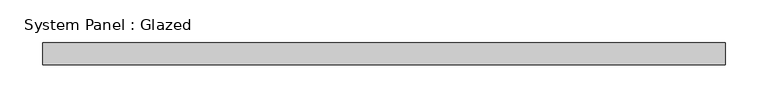
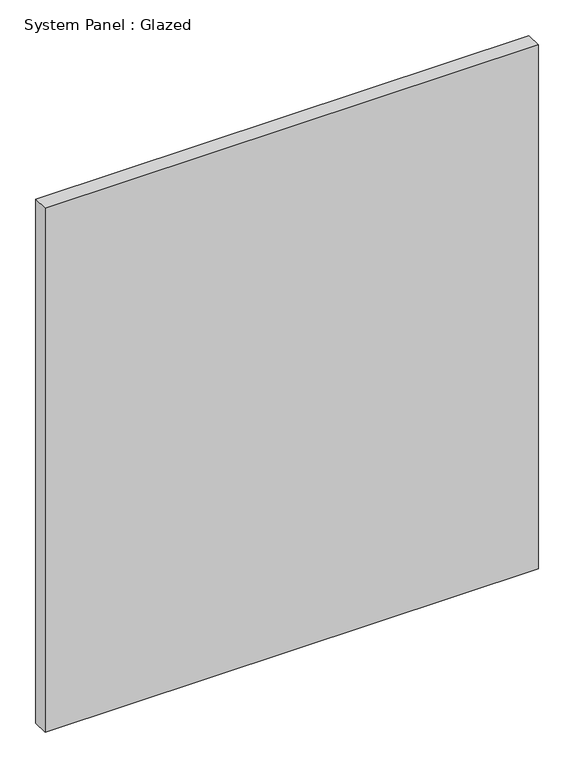
"""IFC4 building model written with IfcOpenShell, lengths in millimetres: plate geometry, System Panel : Glazed."""

from ifc_helpers import new_model, si_unit, origin, origin_with_axes, place, context, project, spatial, polyline, outline, extrude, source, transform, mapped, element, save


def system_panel_glazed_38c9bce4(model_context):
    return source(origin(), model_context, "Body", "SweptSolid", [
        extrude(outline(polyline([(396.875, 19.05), (-396.875, 19.05), (-396.875, 44.45), (396.875, 44.45), (396.875, 19.05)])), origin_with_axes(), (0.0, 0.0, 1.0), 890.5158113),
    ])


if __name__ == "__main__":
    model = new_model("IFC4")
    model_context = context("Model", 3, world=origin())
    ifc_project = project(units=[si_unit("LENGTHUNIT", "METRE", prefix="MILLI")], contexts=[model_context])
    site = spatial("IfcSite", under=ifc_project)
    building = spatial("IfcBuilding", under=site)
    placement = place(None, origin())
    system_panel_glazed_shape = system_panel_glazed_38c9bce4(model_context)
    element("IfcPlate", 1, ObjectType="System Panel : Glazed", at=placement, inside=building, context=model_context, shape_type="MappedRepresentation", body=[
        mapped(system_panel_glazed_shape, transform((0.0, 0.0, 0.0), x_axis=(1.0, 0.0, 0.0), y_axis=(0.0, 1.0, 0.0), z_axis=(0.0, 0.0, 1.0))),
    ])
    save(model, "model.ifc")

# Revit data of these elements
# Type "System Panel : Glazed"
#   Construction Type Id = "GSP4R"
#   Analytic Construction = "1/8 in Pilkington single glazing"
#   Visual Light Transmittance = 0.9
#   Solar Heat Gain Coefficient = 0.86
#   Heat Transfer Coefficient (U) = 1.18115 BTU/(h·ft²·°F)
#   Define Thermal Properties by = 1
# Element 1 (IfcPlate, "System Panel : Glazed")
#   Materials on its faces: "Glass"
# Materials
#   "Glass": class "Glass", colour RGB 0 128 192, transparency 0.75, Description = "Soda Lime Glass", Cost = 0
